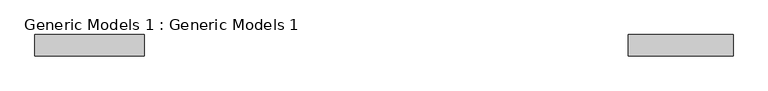
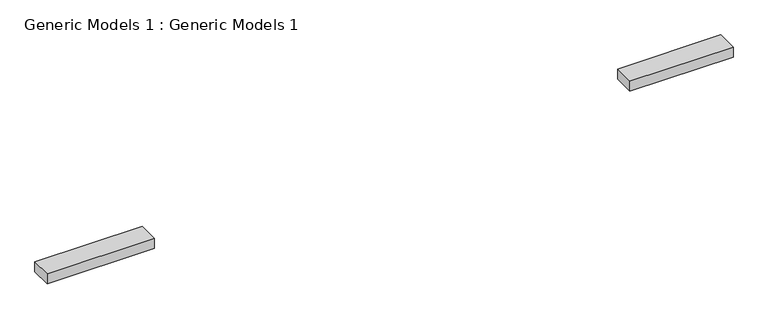
"""IFC4 building model written with IfcOpenShell, lengths in millimetres: proxy geometry, Generic Models 1 : Generic Models 1."""

from ifc_helpers import new_model, si_unit, frame, origin, place, context, project, spatial, polyline, outline, extrude, source, transform, mapped, element, save


def generic_models_1_generic_models_1_2a4bce15(model_context):
    return source(origin(), model_context, "Body", "SweptSolid", [
        extrude(outline(polyline([(-4635.1670283, -6837.0727897), (-6122.6771954, -6837.0727897), (-6122.6771954, -6532.2727897), (-4635.1670283, -6532.2727897), (-4635.1670283, -6837.0727897)])), frame((0.0, 0.0, 2260.6), z_axis=(0.0, 0.0, 1.0), x_axis=(1.0, 0.0, 0.0)), (0.0, 0.0, 1.0), 152.4),
        extrude(outline(polyline([(-12974.453029, -6837.0727897), (-14521.3088608, -6837.0727897), (-14521.3088608, -6532.2727897), (-12974.453029, -6532.2727897), (-12974.453029, -6837.0727897)])), frame((0.0, 0.0, 2260.6), z_axis=(0.0, 0.0, 1.0), x_axis=(1.0, 0.0, 0.0)), (0.0, 0.0, 1.0), 152.4),
    ])


if __name__ == "__main__":
    model = new_model("IFC4")
    model_context = context("Model", 3, world=origin())
    ifc_project = project(units=[si_unit("LENGTHUNIT", "METRE", prefix="MILLI")], contexts=[model_context])
    site = spatial("IfcSite", under=ifc_project)
    building = spatial("IfcBuilding", under=site)
    placement = place(None, origin())
    generic_models_1_generic_models_1_shape = generic_models_1_generic_models_1_2a4bce15(model_context)
    element("IfcBuildingElementProxy", 1, Name="Generic Models 1 : Generic Models 1", ObjectType="Generic Models 1 : Generic Models 1", at=placement, inside=building, context=model_context, shape_type="MappedRepresentation", body=[
        mapped(generic_models_1_generic_models_1_shape, transform((0.0, 0.0, 0.0), x_axis=(1.0, 0.0, 0.0), y_axis=(0.0, 1.0, 0.0), z_axis=(0.0, 0.0, 1.0))),
    ])
    save(model, "model.ifc")
